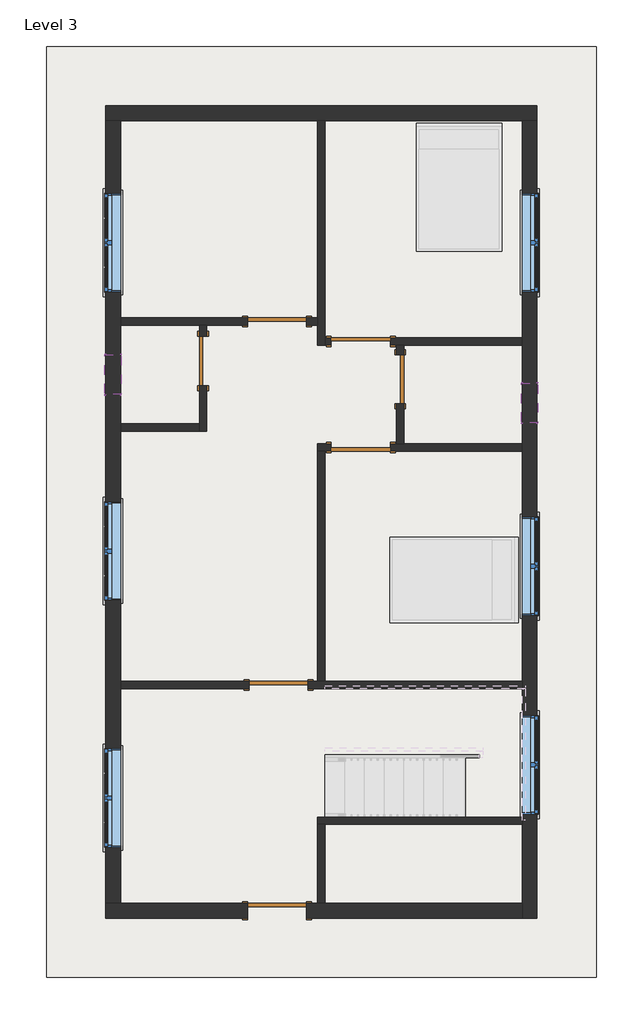
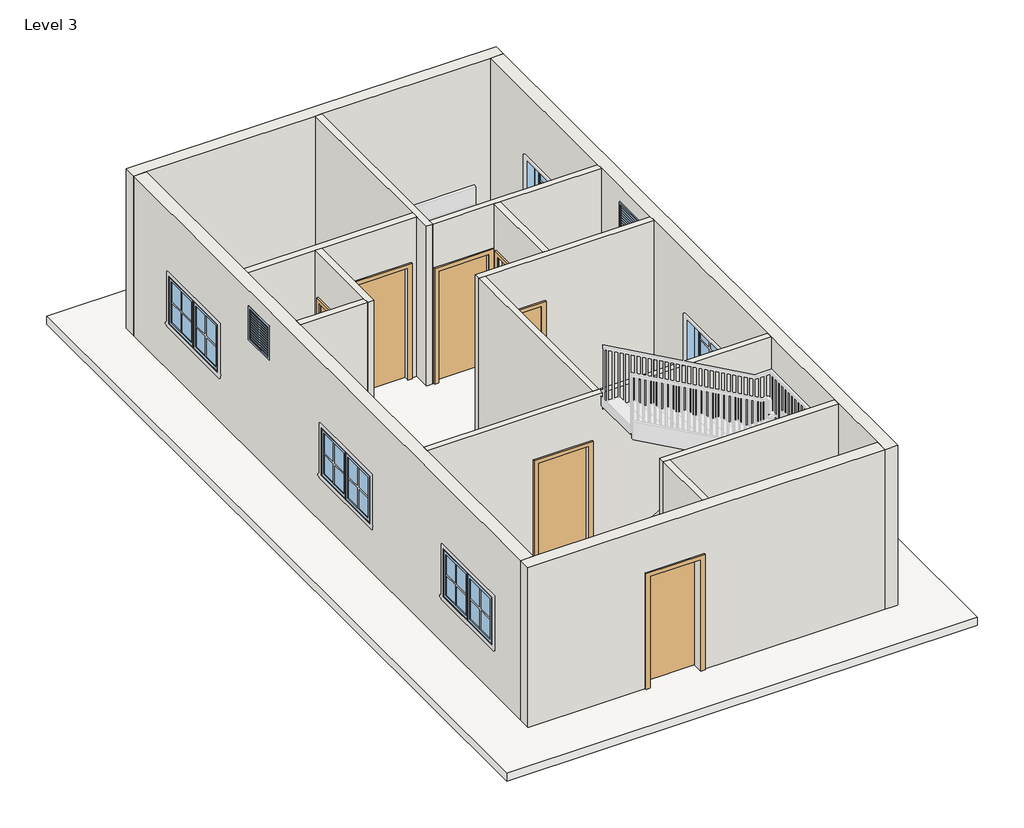
# One storey, part 1 of 3: 15 walls, 8 windows, 7 doors, 1 roof.
"""IFC4 building model written with IfcOpenShell, lengths in millimetres."""

from ifc_helpers import new_model, si_unit, frame, origin, place, context, project, spatial, polyline, outline, extrude, faceted_brep, transform, mapped, element, save
from components import door_78caadf7, door_214872d5, single_flush_door_3_e5f9f3c4, single_flush_door_3_305aa2a5, single_flush_door_3_0ca8825f, window_casement_double_win_5_c1d95f0f, window_f2d8fef0

model = new_model("IFC4")

# Units and contexts
model_context = context("Model", 3, world=origin())
ifc_project = project(units=[si_unit("LENGTHUNIT", "METRE", prefix="MILLI")], contexts=[model_context])

# Site, building, storey
site = spatial("IfcSite", under=ifc_project)
building = spatial("IfcBuilding", under=site)
storey = spatial("IfcBuildingStorey", under=building, Name="Level 3", Elevation=6248.4)

# Doors
placement = place(None, origin())
door_shape = door_78caadf7(model_context)
element("IfcDoor", 1, ObjectType="Single-Flush : 2'6\"", at=placement, inside=storey, context=model_context, shape_type="MappedRepresentation", body=[
    mapped(door_shape, transform((-35.92188, 1946.24131, 6248.4), x_axis=(0.0, 1.0, 0.0), y_axis=(-1.0, 0.0, 0.0), z_axis=(0.0, 0.0, 1.0))),
])
door_2_shape = door_214872d5(model_context)
element("IfcDoor", 2, ObjectType="Single-Flush : 2'6\"", at=placement, inside=storey, context=model_context, shape_type="MappedRepresentation", body=[
    mapped(door_2_shape, transform((-3083.92188, 2225.64131, 6248.4), x_axis=(0.0, 1.0, 0.0), y_axis=(-1.0, 0.0, 0.0), z_axis=(0.0, 0.0, 1.0))),
])
single_flush_door_3_shape = single_flush_door_3_e5f9f3c4(model_context)
element("IfcDoor", 3, ObjectType="Single-Flush : DOOR 3'", at=placement, inside=storey, context=model_context, shape_type="MappedRepresentation", body=[
    mapped(single_flush_door_3_shape, transform((-1940.92188, 2835.24131, 6248.4), x_axis=(1.0, 0.0, 0.0), y_axis=(0.0, 1.0, 0.0), z_axis=(0.0, 0.0, 1.0))),
])
element("IfcDoor", 4, ObjectType="Single-Flush : DOOR 3'", at=placement, inside=storey, context=model_context, shape_type="MappedRepresentation", body=[
    mapped(single_flush_door_3_shape, transform((-645.52188, 892.14131, 6248.4), x_axis=(-1.0, 0.0, 0.0), y_axis=(0.0, -1.0, 0.0), z_axis=(0.0, 0.0, 1.0))),
])
element("IfcDoor", 5, ObjectType="Single-Flush : DOOR 3'", at=placement, inside=storey, context=model_context, shape_type="MappedRepresentation", body=[
    mapped(single_flush_door_3_shape, transform((-1915.52188, -2778.15869, 6248.4), x_axis=(1.0, 0.0, 0.0), y_axis=(0.0, 1.0, 0.0), z_axis=(0.0, 0.0, 1.0))),
])
single_flush_door_3_2_shape = single_flush_door_3_305aa2a5(model_context)
element("IfcDoor", 6, ObjectType="Single-Flush : DOOR 3'", at=placement, inside=storey, context=model_context, shape_type="MappedRepresentation", body=[
    mapped(single_flush_door_3_2_shape, transform((-645.52188, 2530.44131, 6248.4), x_axis=(-1.0, 0.0, 0.0), y_axis=(0.0, -1.0, 0.0), z_axis=(0.0, 0.0, 1.0))),
])
single_flush_door_3_3_shape = single_flush_door_3_0ca8825f(model_context)
element("IfcDoor", 7, ObjectType="Single-Flush : DOOR 3'", at=placement, inside=storey, context=model_context, shape_type="MappedRepresentation", body=[
    mapped(single_flush_door_3_3_shape, transform((-1940.92188, -6264.30869, 6248.4), x_axis=(1.0, 0.0, 0.0), y_axis=(0.0, 1.0, 0.0), z_axis=(0.0, 0.0, 1.0))),
])

# Roof
element("IfcRoof", 8, ObjectType="ROOF 6\"", at=placement, inside=storey, context=model_context, shape_type="SweptSolid", body=[
    extrude(outline(polyline([(-5503.27188, 7083.39131), (2993.02812, 7083.39131), (2993.02812, -7293.00869), (-5503.27188, -7293.00869), (-5503.27188, 7083.39131)])), frame((0.0, 0.0, 6096.0), z_axis=(0.0, 0.0, 1.0), x_axis=(1.0, 0.0, 0.0)), (0.0, 0.0, 1.0), 152.4),
])

# Walls
element("IfcWall", 9, ObjectType="WALL 4.5'", at=placement, inside=storey, context=model_context, shape_type="Brep", body=[
    faceted_brep([(-1312.27188, 5940.39131, 6248.4), (-1312.27188, 2892.39131, 6248.4), (-1312.27188, 2778.09131, 6248.4), (-1312.27188, 2473.29131, 6248.4), (-1312.27188, 2473.29131, 9296.4), (-1312.27188, 2778.09131, 9296.4), (-1312.27188, 2892.39131, 9296.4), (-1312.27188, 5940.39131, 9296.4), (-1197.97188, 5940.39131, 6248.4), (-1197.97188, 5940.39131, 9296.4), (-1197.97188, 2587.59131, 9296.4), (-1197.97188, 2473.29131, 9296.4), (-1197.97188, 2473.29131, 6248.4), (-1197.97188, 2587.59131, 6248.4)], [[[0, 1, 2, 3, 4, 5, 6, 7]], [[8, 9, 10, 11, 12, 13]], [[3, 2, 1, 0, 8, 13, 12]], [[0, 7, 9, 8]], [[4, 3, 12, 11]], [[7, 6, 5, 4, 11, 10, 9]]]),
])
element("IfcWall", 10, ObjectType="WALL 4.5'", at=placement, inside=storey, context=model_context, shape_type="Brep", body=[
    faceted_brep([(-1197.97188, 2473.29131, 6248.4), (-1102.72188, 2473.29131, 6248.4), (-1102.72188, 2473.29131, 8382.0), (-188.32188, 2473.29131, 8382.0), (-188.32188, 2473.29131, 6248.4), (-93.07188, 2473.29131, 6248.4), (21.22812, 2473.29131, 6248.4), (1850.02812, 2473.29131, 6248.4), (1850.02812, 2473.29131, 9296.4), (21.22812, 2473.29131, 9296.4), (-93.07188, 2473.29131, 9296.4), (-1197.97188, 2473.29131, 9296.4), (-1102.72188, 2587.59131, 8382.0), (-1102.72188, 2587.59131, 6248.4), (-1197.97188, 2587.59131, 6248.4), (-1197.97188, 2587.59131, 9296.4), (1850.02812, 2587.59131, 9296.4), (1850.02812, 2587.59131, 6248.4), (-188.32188, 2587.59131, 6248.4), (-188.32188, 2587.59131, 8382.0)], [[[0, 1, 2, 3, 4, 5, 6, 7, 8, 9, 10, 11]], [[12, 13, 14, 15, 16, 17, 18, 19]], [[18, 17, 7, 6, 5, 4]], [[14, 13, 1, 0]], [[0, 11, 15, 14]], [[8, 7, 17, 16]], [[2, 1, 13, 12]], [[3, 2, 12, 19]], [[4, 3, 19, 18]], [[11, 10, 9, 8, 16, 15]]]),
])
element("IfcWall", 11, ObjectType="WALL 4.5'", at=placement, inside=storey, context=model_context, shape_type="Brep", body=[
    faceted_brep([(-1312.27188, 2892.39131, 6248.4), (-1483.72188, 2892.39131, 6248.4), (-1483.72188, 2892.39131, 8382.0), (-2398.12188, 2892.39131, 8382.0), (-2398.12188, 2892.39131, 6248.4), (-4360.27188, 2892.39131, 6248.4), (-4360.27188, 2892.39131, 9296.4), (-1312.27188, 2892.39131, 9296.4), (-1483.72188, 2778.09131, 8382.0), (-1483.72188, 2778.09131, 6248.4), (-1312.27188, 2778.09131, 6248.4), (-1312.27188, 2778.09131, 9296.4), (-3026.77188, 2778.09131, 9296.4), (-3141.07188, 2778.09131, 9296.4), (-4360.27188, 2778.09131, 9296.4), (-4360.27188, 2778.09131, 6248.4), (-3141.07188, 2778.09131, 6248.4), (-3026.77188, 2778.09131, 6248.4), (-2398.12188, 2778.09131, 6248.4), (-2398.12188, 2778.09131, 8382.0)], [[[0, 1, 2, 3, 4, 5, 6, 7]], [[8, 9, 10, 11, 12, 13, 14, 15, 16, 17, 18, 19]], [[10, 9, 1, 0]], [[18, 17, 16, 15, 5, 4]], [[6, 5, 15, 14]], [[0, 7, 11, 10]], [[2, 1, 9, 8]], [[3, 2, 8, 19]], [[4, 3, 19, 18]], [[7, 6, 14, 13, 12, 11]]]),
])
element("IfcWall", 12, ObjectType="WALL 4.5'", at=placement, inside=storey, context=model_context, shape_type="Brep", body=[
    faceted_brep([(-3141.07188, 2778.09131, 6248.4), (-3141.07188, 2606.64131, 6248.4), (-3141.07188, 2606.64131, 8382.0), (-3141.07188, 1844.64131, 8382.0), (-3141.07188, 1844.64131, 6248.4), (-3141.07188, 1254.09131, 6248.4), (-3141.07188, 1139.79131, 6248.4), (-3141.07188, 1139.79131, 9296.4), (-3141.07188, 1254.09131, 9296.4), (-3141.07188, 2778.09131, 9296.4), (-3026.77188, 2606.64131, 8382.0), (-3026.77188, 2606.64131, 6248.4), (-3026.77188, 2778.09131, 6248.4), (-3026.77188, 2778.09131, 9296.4), (-3026.77188, 1139.79131, 9296.4), (-3026.77188, 1139.79131, 6248.4), (-3026.77188, 1844.64131, 6248.4), (-3026.77188, 1844.64131, 8382.0)], [[[0, 1, 2, 3, 4, 5, 6, 7, 8, 9]], [[10, 11, 12, 13, 14, 15, 16, 17]], [[16, 15, 6, 5, 4]], [[12, 11, 1, 0]], [[0, 9, 13, 12]], [[7, 6, 15, 14]], [[2, 1, 11, 10]], [[3, 2, 10, 17]], [[4, 3, 17, 16]], [[9, 8, 7, 14, 13]]]),
])
element("IfcWall", 13, ObjectType="WALL 4.5'", at=placement, inside=storey, context=model_context, shape_type="SweptSolid", body=[
    extrude(outline(polyline([(-4360.27188, 1254.09131), (-3141.07188, 1254.09131), (-3141.07188, 1139.79131), (-4360.27188, 1139.79131), (-4360.27188, 1254.09131)])), frame((0.0, 0.0, 6248.4), z_axis=(0.0, 0.0, 1.0), x_axis=(1.0, 0.0, 0.0)), (0.0, 0.0, 1.0), 3048.0),
])
element("IfcWall", 14, ObjectType="WALL 4.5'", at=placement, inside=storey, context=model_context, shape_type="SweptSolid", body=[
    extrude(outline(polyline([(2473.29131, 6248.4), (2327.24131, 6248.4), (2327.24131, 8382.0), (1565.24131, 8382.0), (1565.24131, 6248.4), (949.29131, 6248.4), (949.29131, 9296.4), (2473.29131, 9296.4), (2473.29131, 6248.4)])), frame((-93.07188, 0.0, 0.0), z_axis=(1.0, 0.0, 0.0), x_axis=(0.0, 1.0, 0.0)), (0.0, 0.0, 1.0), 114.3),
])
element("IfcWall", 15, ObjectType="WALL 4.5'", at=placement, inside=storey, context=model_context, shape_type="Brep", body=[
    faceted_brep([(-1102.72188, 949.29131, 8382.0), (-1102.72188, 949.29131, 6248.4), (-1312.27188, 949.29131, 6248.4), (-1312.27188, 949.29131, 9296.4), (-93.07188, 949.29131, 9296.4), (21.22812, 949.29131, 9296.4), (1850.02812, 949.29131, 9296.4), (1850.02812, 949.29131, 6248.4), (21.22812, 949.29131, 6248.4), (-93.07188, 949.29131, 6248.4), (-188.32188, 949.29131, 6248.4), (-188.32188, 949.29131, 8382.0), (-1312.27188, 834.99131, 6248.4), (-1197.97188, 834.99131, 6248.4), (-1102.72188, 834.99131, 6248.4), (-1102.72188, 834.99131, 8382.0), (-188.32188, 834.99131, 8382.0), (-188.32188, 834.99131, 6248.4), (1850.02812, 834.99131, 6248.4), (1850.02812, 834.99131, 9296.4), (-1197.97188, 834.99131, 9296.4), (-1312.27188, 834.99131, 9296.4)], [[[0, 1, 2, 3, 4, 5, 6, 7, 8, 9, 10, 11]], [[12, 13, 14, 15, 16, 17, 18, 19, 20, 21]], [[2, 1, 14, 13, 12]], [[10, 9, 8, 7, 18, 17]], [[7, 6, 19, 18]], [[3, 2, 12, 21]], [[15, 14, 1, 0]], [[16, 15, 0, 11]], [[17, 16, 11, 10]], [[6, 5, 4, 3, 21, 20, 19]]]),
])
element("IfcWall", 16, ObjectType="WALL 4.5'", at=placement, inside=storey, context=model_context, shape_type="SweptSolid", body=[
    extrude(outline(polyline([(-1312.27188, -2721.00869), (-1312.27188, 834.99131), (-1197.97188, 834.99131), (-1197.97188, -2721.00869), (-1312.27188, -2721.00869)])), frame((0.0, 0.0, 6248.4), z_axis=(0.0, 0.0, 1.0), x_axis=(1.0, 0.0, 0.0)), (0.0, 0.0, 1.0), 3048.0),
])
element("IfcWall", 17, ObjectType="WALL 4.5'", at=placement, inside=storey, context=model_context, shape_type="Brep", body=[
    faceted_brep([(1850.02812, -2721.00869, 6248.4), (-1197.97188, -2721.00869, 6248.4), (-1312.27188, -2721.00869, 6248.4), (-1458.32188, -2721.00869, 6248.4), (-1458.32188, -2721.00869, 8382.0), (-2372.72188, -2721.00869, 8382.0), (-2372.72188, -2721.00869, 6248.4), (-4360.27188, -2721.00869, 6248.4), (-4360.27188, -2721.00869, 9296.4), (-1312.27188, -2721.00869, 9296.4), (-1197.97188, -2721.00869, 9296.4), (1850.02812, -2721.00869, 9296.4), (-1458.32188, -2835.30869, 8382.0), (-1458.32188, -2835.30869, 6248.4), (1850.02812, -2835.30869, 6248.4), (1850.02812, -2835.30869, 9296.4), (-4360.27188, -2835.30869, 9296.4), (-4360.27188, -2835.30869, 6248.4), (-2372.72188, -2835.30869, 6248.4), (-2372.72188, -2835.30869, 8382.0)], [[[0, 1, 2, 3, 4, 5, 6, 7, 8, 9, 10, 11]], [[12, 13, 14, 15, 16, 17, 18, 19]], [[18, 17, 7, 6]], [[14, 13, 3, 2, 1, 0]], [[0, 11, 15, 14]], [[8, 7, 17, 16]], [[4, 3, 13, 12]], [[5, 4, 12, 19]], [[6, 5, 19, 18]], [[11, 10, 9, 8, 16, 15]]]),
])
element("IfcWall", 18, ObjectType="WALL 4.5'", at=placement, inside=storey, context=model_context, shape_type="Brep", body=[
    faceted_brep([(1850.02812, -4816.50869, 6248.4), (-1312.27188, -4816.50869, 6248.4), (-1312.27188, -4816.50869, 9296.4), (1850.02812, -4816.50869, 9296.4), (1850.02812, -4930.80869, 6248.4), (1850.02812, -4930.80869, 9296.4), (-1197.97188, -4930.80869, 9296.4), (-1312.27188, -4930.80869, 9296.4), (-1312.27188, -4930.80869, 6248.4), (-1197.97188, -4930.80869, 6248.4)], [[[0, 1, 2, 3]], [[4, 5, 6, 7, 8, 9]], [[1, 0, 4, 9, 8]], [[0, 3, 5, 4]], [[2, 1, 8, 7]], [[3, 2, 7, 6, 5]]]),
])
element("IfcWall", 19, ObjectType="WALL 4.5'", at=placement, inside=storey, context=model_context, shape_type="SweptSolid", body=[
    extrude(outline(polyline([(-1312.27188, -6150.00869), (-1312.27188, -4930.80869), (-1197.97188, -4930.80869), (-1197.97188, -6150.00869), (-1312.27188, -6150.00869)])), frame((0.0, 0.0, 6248.4), z_axis=(0.0, 0.0, 1.0), x_axis=(1.0, 0.0, 0.0)), (0.0, 0.0, 1.0), 3048.0),
])
element("IfcWall", 20, ObjectType="WALL 9\"", at=placement, inside=storey, context=model_context, shape_type="Brep", body=[
    faceted_brep([(-4588.87188, 5940.39131, 6248.4), (-4360.27188, 5940.39131, 6248.4), (-1312.27188, 5940.39131, 6248.4), (-1197.97188, 5940.39131, 6248.4), (1850.02812, 5940.39131, 6248.4), (2078.62812, 5940.39131, 6248.4), (2078.62812, 5940.39131, 9296.4), (1850.02812, 5940.39131, 9296.4), (-1197.97188, 5940.39131, 9296.4), (-1312.27188, 5940.39131, 9296.4), (-4360.27188, 5940.39131, 9296.4), (-4588.87188, 5940.39131, 9296.4), (-4588.87188, 6168.99131, 6248.4), (-4588.87188, 6168.99131, 9296.4), (2078.62812, 6168.99131, 9296.4), (2078.62812, 6168.99131, 6248.4)], [[[0, 1, 2, 3, 4, 5, 6, 7, 8, 9, 10, 11]], [[12, 13, 14, 15]], [[5, 4, 3, 2, 1, 0, 12, 15]], [[6, 5, 15, 14]], [[0, 11, 13, 12]], [[11, 10, 9, 8, 7, 6, 14, 13]]]),
])
element("IfcWall", 21, ObjectType="WALL 9\"", at=placement, inside=storey, context=model_context, shape_type="Brep", body=[
    faceted_brep([(1850.02812, 5940.39131, 6248.4), (1850.02812, 2587.59131, 6248.4), (1850.02812, 2473.29131, 6248.4), (1850.02812, 949.29131, 6248.4), (1850.02812, 834.99131, 6248.4), (1850.02812, -2721.00869, 6248.4), (1850.02812, -2835.30869, 6248.4), (1850.02812, -4816.50869, 6248.4), (1850.02812, -4930.80869, 6248.4), (1850.02812, -6150.00869, 6248.4), (1850.02812, -6378.60869, 6248.4), (1850.02812, -6378.60869, 9296.4), (1850.02812, -6150.00869, 9296.4), (1850.02812, -4930.80869, 9296.4), (1850.02812, -4816.50869, 9296.4), (1850.02812, -2835.30869, 9296.4), (1850.02812, -2721.00869, 9296.4), (1850.02812, 834.99131, 9296.4), (1850.02812, 949.29131, 9296.4), (1850.02812, 2473.29131, 9296.4), (1850.02812, 2587.59131, 9296.4), (1850.02812, 5940.39131, 9296.4), (1850.02812, -4772.05869, 8077.2), (1850.02812, -4772.05869, 7162.8), (1850.02812, -3248.05869, 7162.8), (1850.02812, -3248.05869, 8077.2), (1850.02812, 3292.44131, 8077.2), (1850.02812, 3292.44131, 7162.8), (1850.02812, 4816.44131, 7162.8), (1850.02812, 4816.44131, 8077.2), (1850.02812, -1705.00869, 8077.2), (1850.02812, -1705.00869, 7162.8), (1850.02812, -181.00869, 7162.8), (1850.02812, -181.00869, 8077.2), (1850.02812, 1273.14131, 8991.6), (1850.02812, 1273.14131, 8382.0), (1850.02812, 1882.74131, 8382.0), (1850.02812, 1882.74131, 8991.6), (2078.62812, 5940.39131, 6248.4), (2078.62812, 5940.39131, 9296.4), (2078.62812, -6378.60869, 9296.4), (2078.62812, -6378.60869, 6248.4), (2078.62812, -4772.05869, 8077.2), (2078.62812, -3248.05869, 8077.2), (2078.62812, -3248.05869, 7162.8), (2078.62812, -4772.05869, 7162.8), (2078.62812, 3292.44131, 8077.2), (2078.62812, 4816.44131, 8077.2), (2078.62812, 4816.44131, 7162.8), (2078.62812, 3292.44131, 7162.8), (2078.62812, -1705.00869, 8077.2), (2078.62812, -181.00869, 8077.2), (2078.62812, -181.00869, 7162.8), (2078.62812, -1705.00869, 7162.8), (2078.62812, 1273.14131, 8991.6), (2078.62812, 1882.74131, 8991.6), (2078.62812, 1882.74131, 8382.0), (2078.62812, 1273.14131, 8382.0)], [[[0, 1, 2, 3, 4, 5, 6, 7, 8, 9, 10, 11, 12, 13, 14, 15, 16, 17, 18, 19, 20, 21], [22, 23, 24, 25], [26, 27, 28, 29], [30, 31, 32, 33], [34, 35, 36, 37]], [[38, 39, 40, 41], [42, 43, 44, 45], [46, 47, 48, 49], [50, 51, 52, 53], [54, 55, 56, 57]], [[10, 9, 8, 7, 6, 5, 4, 3, 2, 1, 0, 38, 41]], [[0, 21, 39, 38]], [[11, 10, 41, 40]], [[23, 22, 42, 45]], [[24, 23, 45, 44]], [[25, 24, 44, 43]], [[22, 25, 43, 42]], [[27, 26, 46, 49]], [[28, 27, 49, 48]], [[29, 28, 48, 47]], [[26, 29, 47, 46]], [[31, 30, 50, 53]], [[32, 31, 53, 52]], [[33, 32, 52, 51]], [[30, 33, 51, 50]], [[35, 34, 54, 57]], [[36, 35, 57, 56]], [[37, 36, 56, 55]], [[34, 37, 55, 54]], [[21, 20, 19, 18, 17, 16, 15, 14, 13, 12, 11, 40, 39]]]),
])
element("IfcWall", 22, ObjectType="WALL 9\"", at=placement, inside=storey, context=model_context, shape_type="Brep", body=[
    faceted_brep([(1850.02812, -6150.00869, 6248.4), (-1197.97188, -6150.00869, 6248.4), (-1312.27188, -6150.00869, 6248.4), (-1483.72188, -6150.00869, 6248.4), (-1483.72188, -6150.00869, 8382.0), (-2398.12188, -6150.00869, 8382.0), (-2398.12188, -6150.00869, 6248.4), (-4360.27188, -6150.00869, 6248.4), (-4588.87188, -6150.00869, 6248.4), (-4588.87188, -6150.00869, 9296.4), (-4360.27188, -6150.00869, 9296.4), (-1312.27188, -6150.00869, 9296.4), (-1197.97188, -6150.00869, 9296.4), (1850.02812, -6150.00869, 9296.4), (-1483.72188, -6378.60869, 8382.0), (-1483.72188, -6378.60869, 6248.4), (1850.02812, -6378.60869, 6248.4), (1850.02812, -6378.60869, 9296.4), (-4588.87188, -6378.60869, 9296.4), (-4588.87188, -6378.60869, 6248.4), (-2398.12188, -6378.60869, 6248.4), (-2398.12188, -6378.60869, 8382.0)], [[[0, 1, 2, 3, 4, 5, 6, 7, 8, 9, 10, 11, 12, 13]], [[14, 15, 16, 17, 18, 19, 20, 21]], [[20, 19, 8, 7, 6]], [[16, 15, 3, 2, 1, 0]], [[0, 13, 17, 16]], [[9, 8, 19, 18]], [[4, 3, 15, 14]], [[5, 4, 14, 21]], [[6, 5, 21, 20]], [[13, 12, 11, 10, 9, 18, 17]]]),
])
element("IfcWall", 23, ObjectType="WALL 9\"", at=placement, inside=storey, context=model_context, shape_type="Brep", body=[
    faceted_brep([(-4360.27188, -6150.00869, 6248.4), (-4360.27188, -2835.30869, 6248.4), (-4360.27188, -2721.00869, 6248.4), (-4360.27188, 1139.79131, 6248.4), (-4360.27188, 1254.09131, 6248.4), (-4360.27188, 2778.09131, 6248.4), (-4360.27188, 2892.39131, 6248.4), (-4360.27188, 5940.39131, 6248.4), (-4360.27188, 5940.39131, 9296.4), (-4360.27188, 2892.39131, 9296.4), (-4360.27188, 2778.09131, 9296.4), (-4360.27188, 1254.09131, 9296.4), (-4360.27188, 1139.79131, 9296.4), (-4360.27188, -2721.00869, 9296.4), (-4360.27188, -2835.30869, 9296.4), (-4360.27188, -6150.00869, 9296.4), (-4360.27188, 4816.44131, 8077.2), (-4360.27188, 4816.44131, 7162.8), (-4360.27188, 3292.44131, 7162.8), (-4360.27188, 3292.44131, 8077.2), (-4360.27188, 53.94131, 8077.2), (-4360.27188, 53.94131, 7162.8), (-4360.27188, -1470.05869, 7162.8), (-4360.27188, -1470.05869, 8077.2), (-4360.27188, -3759.23369, 8077.2), (-4360.27188, -3759.23369, 7162.8), (-4360.27188, -5283.23369, 7162.8), (-4360.27188, -5283.23369, 8077.2), (-4360.27188, 1711.29131, 8991.6), (-4360.27188, 2320.89131, 8991.6), (-4360.27188, 2320.89131, 8382.0), (-4360.27188, 1711.29131, 8382.0), (-4588.87188, -6150.00869, 6248.4), (-4588.87188, -6150.00869, 9296.4), (-4588.87188, 5940.39131, 9296.4), (-4588.87188, 5940.39131, 6248.4), (-4588.87188, 4816.44131, 8077.2), (-4588.87188, 3292.44131, 8077.2), (-4588.87188, 3292.44131, 7162.8), (-4588.87188, 4816.44131, 7162.8), (-4588.87188, 53.94131, 8077.2), (-4588.87188, -1470.05869, 8077.2), (-4588.87188, -1470.05869, 7162.8), (-4588.87188, 53.94131, 7162.8), (-4588.87188, -3759.23369, 8077.2), (-4588.87188, -5283.23369, 8077.2), (-4588.87188, -5283.23369, 7162.8), (-4588.87188, -3759.23369, 7162.8), (-4588.87188, 1711.29131, 8991.6), (-4588.87188, 1711.29131, 8382.0), (-4588.87188, 2320.89131, 8382.0), (-4588.87188, 2320.89131, 8991.6)], [[[0, 1, 2, 3, 4, 5, 6, 7, 8, 9, 10, 11, 12, 13, 14, 15], [16, 17, 18, 19], [20, 21, 22, 23], [24, 25, 26, 27], [28, 29, 30, 31]], [[32, 33, 34, 35], [36, 37, 38, 39], [40, 41, 42, 43], [44, 45, 46, 47], [48, 49, 50, 51]], [[7, 6, 5, 4, 3, 2, 1, 0, 32, 35]], [[8, 7, 35, 34]], [[0, 15, 33, 32]], [[17, 16, 36, 39]], [[18, 17, 39, 38]], [[19, 18, 38, 37]], [[16, 19, 37, 36]], [[21, 20, 40, 43]], [[22, 21, 43, 42]], [[23, 22, 42, 41]], [[20, 23, 41, 40]], [[25, 24, 44, 47]], [[26, 25, 47, 46]], [[27, 26, 46, 45]], [[24, 27, 45, 44]], [[49, 48, 28, 31]], [[50, 49, 31, 30]], [[51, 50, 30, 29]], [[48, 51, 29, 28]], [[15, 14, 13, 12, 11, 10, 9, 8, 34, 33]]]),
])

# Windows
window_casement_double_win_5_shape = window_casement_double_win_5_c1d95f0f(model_context)
element("IfcWindow", 24, ObjectType="Window-Casement-Double : WIN 5'", at=placement, inside=storey, context=model_context, shape_type="MappedRepresentation", body=[
    mapped(window_casement_double_win_5_shape, transform((-4474.57188, 4054.44131, 6248.4), x_axis=(0.0, 1.0, 0.0), y_axis=(-1.0, 0.0, 0.0), z_axis=(0.0, 0.0, 1.0))),
])
element("IfcWindow", 25, ObjectType="Window-Casement-Double : WIN 5'", at=placement, inside=storey, context=model_context, shape_type="MappedRepresentation", body=[
    mapped(window_casement_double_win_5_shape, transform((-4474.57188, -708.05869, 6248.4), x_axis=(0.0, 1.0, 0.0), y_axis=(-1.0, 0.0, 0.0), z_axis=(0.0, 0.0, 1.0))),
])
element("IfcWindow", 26, ObjectType="Window-Casement-Double : WIN 5'", at=placement, inside=storey, context=model_context, shape_type="MappedRepresentation", body=[
    mapped(window_casement_double_win_5_shape, transform((-4474.57188, -4521.23369, 6248.4), x_axis=(0.0, 1.0, 0.0), y_axis=(-1.0, 0.0, 0.0), z_axis=(0.0, 0.0, 1.0))),
])
element("IfcWindow", 27, ObjectType="Window-Casement-Double : WIN 5'", at=placement, inside=storey, context=model_context, shape_type="MappedRepresentation", body=[
    mapped(window_casement_double_win_5_shape, transform((1964.32812, -4010.05869, 6248.4), x_axis=(0.0, -1.0, 0.0), y_axis=(1.0, 0.0, 0.0), z_axis=(0.0, 0.0, 1.0))),
])
element("IfcWindow", 28, ObjectType="Window-Casement-Double : WIN 5'", at=placement, inside=storey, context=model_context, shape_type="MappedRepresentation", body=[
    mapped(window_casement_double_win_5_shape, transform((1964.32812, 4054.44131, 6248.4), x_axis=(0.0, -1.0, 0.0), y_axis=(1.0, 0.0, 0.0), z_axis=(0.0, 0.0, 1.0))),
])
element("IfcWindow", 29, ObjectType="Window-Casement-Double : WIN 5'", at=placement, inside=storey, context=model_context, shape_type="MappedRepresentation", body=[
    mapped(window_casement_double_win_5_shape, transform((1964.32812, -943.00869, 6248.4), x_axis=(0.0, -1.0, 0.0), y_axis=(1.0, 0.0, 0.0), z_axis=(0.0, 0.0, 1.0))),
])
window_shape = window_f2d8fef0(model_context)
element("IfcWindow", 30, ObjectType="Window-Louvers : 24\" x 24\"", at=placement, inside=storey, context=model_context, shape_type="MappedRepresentation", body=[
    mapped(window_shape, transform((1957.97812, 1577.94131, 7467.6), x_axis=(0.0, 1.0, 0.0), y_axis=(-1.0, 0.0, 0.0), z_axis=(0.0, 0.0, 1.0))),
])
element("IfcWindow", 31, ObjectType="Window-Louvers : 24\" x 24\"", at=placement, inside=storey, context=model_context, shape_type="MappedRepresentation", body=[
    mapped(window_shape, transform((-4480.92188, 2016.09131, 7467.6), x_axis=(0.0, 1.0, 0.0), y_axis=(-1.0, 0.0, 0.0), z_axis=(0.0, 0.0, 1.0))),
])

save(model, "model.ifc")

# Revit data of these elements
# Type "Single-Flush : 2'6\""
#   Type Mark = "9"
#   Construction Type Id = "MDOOR"
#   Assembly Code = "C1020"
#   Analytic Construction = "Metal"
#   Thickness = 0' - 2"
#   Heat Transfer Coefficient (U) = 0.651978 BTU/(h·ft²·°F)
#   Height = 7' - 0"
#   Trim Projection Ext = 0' - 1"
#   Trim Projection Int = 0' - 1"
#   Trim Width = 0' - 3"
#   Width = 2' - 6"
#   Define Thermal Properties by = 1
#   Door Material = Door - Panel
#   Frame Material = Door - Frame
#   Visual Light Transmittance = 0
#   Solar Heat Gain Coefficient = 0
#   Function = (empty or 0)
#   Wall Closure = (empty or 0)
# Type "Single-Flush : DOOR 3'"
#   Type Mark = "8"
#   Construction Type Id = "MDOOR"
#   Assembly Code = "C1020"
#   Analytic Construction = "Metal"
#   Thickness = 0' - 2"
#   Heat Transfer Coefficient (U) = 0.651978 BTU/(h·ft²·°F)
#   Height = 7' - 0"
#   Trim Projection Ext = 0' - 1"
#   Trim Projection Int = 0' - 1"
#   Trim Width = 0' - 3"
#   Width = 3' - 0"
#   Define Thermal Properties by = 1
#   Door Material = Door - Panel
#   Frame Material = Door - Frame
#   Visual Light Transmittance = 0
#   Solar Heat Gain Coefficient = 0
#   Function = (empty or 0)
#   Wall Closure = (empty or 0)
# Type "ROOF 6\""
#   Assembly Code = "B1020"
#   Layers, outside or top first: 0' - 6" no material (function 1)
# Type "WALL 4.5'"
#   Assembly Code = "B2010"
#   Layers, outside or top first: 0' - 4 1/2" no material (function 1)
# Type "WALL 9\""
#   Assembly Code = "B2010"
#   Layers, outside or top first: 0' - 9" no material (function 1)
# Type "Window-Casement-Double : WIN 5'"
#   Type Mark = "18"
#   Fire Rating = "0.5h"
#   Assembly Code = "B2020100"
#   Analytic Construction = "Double glazing - domestic"
#   Frame Extension [instance default] = 0' - 0 1/4"
#   Window Inset [instance default] = 0' - 0"
#   Wall Thickness [instance default] = 0' - 6"
#   Interior Wall Closure [instance default] = 0' - 2 1/4"
#   Half Width = 2' - 6"
#   Visual Light Transmittance = 0.81
#   Thermal Resistance (R) = 1.8146 (h·ft²·°F)/BTU
#   Solar Heat Gain Coefficient = 0.76
#   Rough Width = 5' - 0 1/2"
#   Rough Height = 3' - 0 1/2"
#   Height = 3' - 0"
#   Heat Transfer Coefficient (U) = 0.5511 BTU/(h·ft²·°F)
#   Exterior Wall Closure [instance default] = 0' - 1 1/4"
#   Extension Jamb [instance default] = 0' - 2 1/4"
#   Default Sill Height = 3' - 0"
#   Width = 5' - 0"
#   Muntin Visibility = yes
#   Interior Trim Visibility [instance default] = yes
#   Exterior Trim Visibility [instance default] = yes
#   Extension Jamb Visibility [instance default] = yes
#   Interior Trim Material = Wood - Stained
#   Muntin Pattern = Muntin Pattern_2x2 : Muntin Pattern_2x2
#   Interior Trim = Trim-Window-Interior-Flat : Picture Frame
#   Interior Frame Material = Wood - Stained
#   Glass Panel Material = Glass
#   Exterior Trim Material = Clad - White
#   Exterior Trim = Trim-Window-Exterior-Flat : with Sill
#   Exterior Frame Material = Clad - White
#   Wall Closure = (empty or 0)
# Type "Window-Louvers : 24\" x 24\""
#   Type Mark = "19"
#   Construction Type Id = "GSP4R"
#   Assembly Code = "B20"
#   Analytic Construction = "1/8 in Pilkington single glazing"
#   Visual Light Transmittance = 0.9
#   Thermal Resistance (R) = 1.53941 (h·ft²·°F)/BTU
#   Solar Heat Gain Coefficient = 0.78
#   Max Height = 1' - 11.74264"
#   Height = 2' - 0"
#   Heat Transfer Coefficient (U) = 0.6496 BTU/(h·ft²·°F)
#   Blade Width [instance default] = 1' - 10 1/2"
#   Blade Vertical Thickness = 0' - 0.35355"
#   Blade Thickness = 0' - 0 1/4"
#   Blade Spacing = 0' - 1 1/2"
#   Blade Height = 0' - 1.85355"
#   Blade Depth = 0' - 3"
#   Blade Angle = 45.00°
#   Default Sill Height = 3' - 0"
#   Trim Projection_Exterior = 0' - 0 1/2"
#   Trim Projection_Interior = 0' - 0 1/2"
#   Trim Width_Exterior = 0' - 1 1/2"
#   Trim Width_Interior = 0' - 1 1/2"
#   Width = 2' - 0"
#   Max Blade Count = 12
#   Define Thermal Properties by = 1
#   Blade Count = 12
#   Frame Material = Birch
#   Louver Material = Birch
#   Trim Exterior Material = Birch
#   Trim Interior Material = Birch
#   Wall Closure = (empty or 0)
# Elements 1, 2 (IfcDoor, "Single-Flush : 2'6\"")
#   Phase Created = New Construction
#   Materials on its faces: "Door - Frame", "Door - Panel"
# Elements 3, 4, 5, 6, 7 (IfcDoor, "Single-Flush : DOOR 3'")
#   Phase Created = New Construction
#   Materials on its faces: "Door - Frame", "Door - Panel"
# Element 8 (IfcRoof, "ROOF 6\"")
#   built-in parameter 1001705 = 20.5 (stored number, unit not read)
#   built-in parameter 1001701 = -0.5 (stored number, unit not read)
#   built-in parameter 1001710 = 33615
#   Phase Created = New Construction
#   Materials on its faces: "Parking Stripe", "Default Roof", "Wood - Stained"
# Elements 9, 10, 11, 12, 13, 14, 15, 16, 17, 18, 19 (IfcWall, "WALL 4.5'")
#   Top Offset = 0' - 0"
#   Base Offset = 0' - 0"
#   Unconnected Height = 10' - 0"
#   wall height = 10' - 0"
#   Phase Created = New Construction
#   Base Constraint = Level 3
#   Materials on its faces: "Default Wall"
# Elements 20, 21, 22, 23 (IfcWall, "WALL 9\"")
#   Top Offset = 0' - 0"
#   Base Offset = 0' - 0"
#   Unconnected Height = 10' - 0"
#   wall height = 10' - 0"
#   Phase Created = New Construction
#   Base Constraint = Level 3
#   Materials on its faces: "Default Wall", "Copper"
# Element 24 (IfcWindow, "Window-Casement-Double : WIN 5'")
#   Mark = "17"
#   Window Inset = 0' - 0"
#   Interior Wall Closure = 0' - 2 1/4"
#   Frame Extension = 0' - 0 1/4"
#   Exterior Wall Closure = 0' - 1 1/4"
#   Interior Trim Visibility = yes
#   Exterior Trim Visibility = yes
#   Phase Created = New Construction
#   Materials on its faces: "Wood - Stained", "Glass", "Clad - White"
# Element 25 (IfcWindow, "Window-Casement-Double : WIN 5'")
#   Mark = "18"
#   Window Inset = 0' - 0"
#   Interior Wall Closure = 0' - 2 1/4"
#   Frame Extension = 0' - 0 1/4"
#   Exterior Wall Closure = 0' - 1 1/4"
#   Interior Trim Visibility = yes
#   Exterior Trim Visibility = yes
#   Phase Created = New Construction
#   Materials on its faces: "Wood - Stained", "Glass", "Clad - White"
# Element 26 (IfcWindow, "Window-Casement-Double : WIN 5'")
#   Mark = "19"
#   Window Inset = 0' - 0"
#   Interior Wall Closure = 0' - 2 1/4"
#   Frame Extension = 0' - 0 1/4"
#   Exterior Wall Closure = 0' - 1 1/4"
#   Interior Trim Visibility = yes
#   Exterior Trim Visibility = yes
#   Phase Created = New Construction
#   Materials on its faces: "Wood - Stained", "Glass", "Clad - White"
# Element 27 (IfcWindow, "Window-Casement-Double : WIN 5'")
#   Mark = "20"
#   Window Inset = 0' - 0"
#   Interior Wall Closure = 0' - 2 1/4"
#   Frame Extension = 0' - 0 1/4"
#   Exterior Wall Closure = 0' - 1 1/4"
#   Interior Trim Visibility = yes
#   Exterior Trim Visibility = yes
#   Phase Created = New Construction
#   Materials on its faces: "Wood - Stained", "Glass", "Clad - White"
# Element 28 (IfcWindow, "Window-Casement-Double : WIN 5'")
#   Mark = "21"
#   Window Inset = 0' - 0"
#   Interior Wall Closure = 0' - 2 1/4"
#   Frame Extension = 0' - 0 1/4"
#   Exterior Wall Closure = 0' - 1 1/4"
#   Interior Trim Visibility = yes
#   Exterior Trim Visibility = yes
#   Phase Created = New Construction
#   Materials on its faces: "Wood - Stained", "Glass", "Clad - White"
# Element 29 (IfcWindow, "Window-Casement-Double : WIN 5'")
#   Mark = "22"
#   Window Inset = 0' - 0"
#   Interior Wall Closure = 0' - 2 1/4"
#   Frame Extension = 0' - 0 1/4"
#   Exterior Wall Closure = 0' - 1 1/4"
#   Interior Trim Visibility = yes
#   Exterior Trim Visibility = yes
#   Phase Created = New Construction
#   Materials on its faces: "Wood - Stained", "Glass", "Clad - White"
# Element 30 (IfcWindow, "Window-Louvers : 24\" x 24\"")
#   Mark = "23"
#   Blade Width = 1' - 10 1/2"
#   Phase Created = New Construction
#   Materials on its faces: "Birch"
# Element 31 (IfcWindow, "Window-Louvers : 24\" x 24\"")
#   Mark = "24"
#   Blade Width = 1' - 10 1/2"
#   Phase Created = New Construction
#   Materials on its faces: "Birch"
# Materials
#   "Door - Panel": class "Wood", colour RGB 210 159 95, transparency 0, Cost = 0
#   "Door - Frame": colour RGB 118 70 51, transparency 0, Cost = 0
#   "Wood - Stained": class "Wood", colour RGB 224 178 126, transparency 0, Cost = 0
#   "Glass": class "Glass", colour RGB 0 128 192, transparency 0.75, Description = "Soda Lime Glass", Cost = 0
#   "Clad - White": class "Wood", colour RGB 242 242 238, transparency 0, Cost = 0
#   "Birch": class "Wood", colour RGB 224 178 126, transparency 0, Description = "Betula Alleghaniensis", Cost = 0
#   "Parking Stripe": class "Paint", colour RGB 250 250 91, transparency 0, Cost = 0
#   "Default Roof": colour RGB 88 101 114, transparency 0, Cost = 0
#   "Default Wall": colour RGB 128 128 128, transparency 0, Cost = 0
#   "Copper": class "Metal", colour RGB 0 0 0, transparency 0, Description = "Copper, matte finish", Cost = 0
